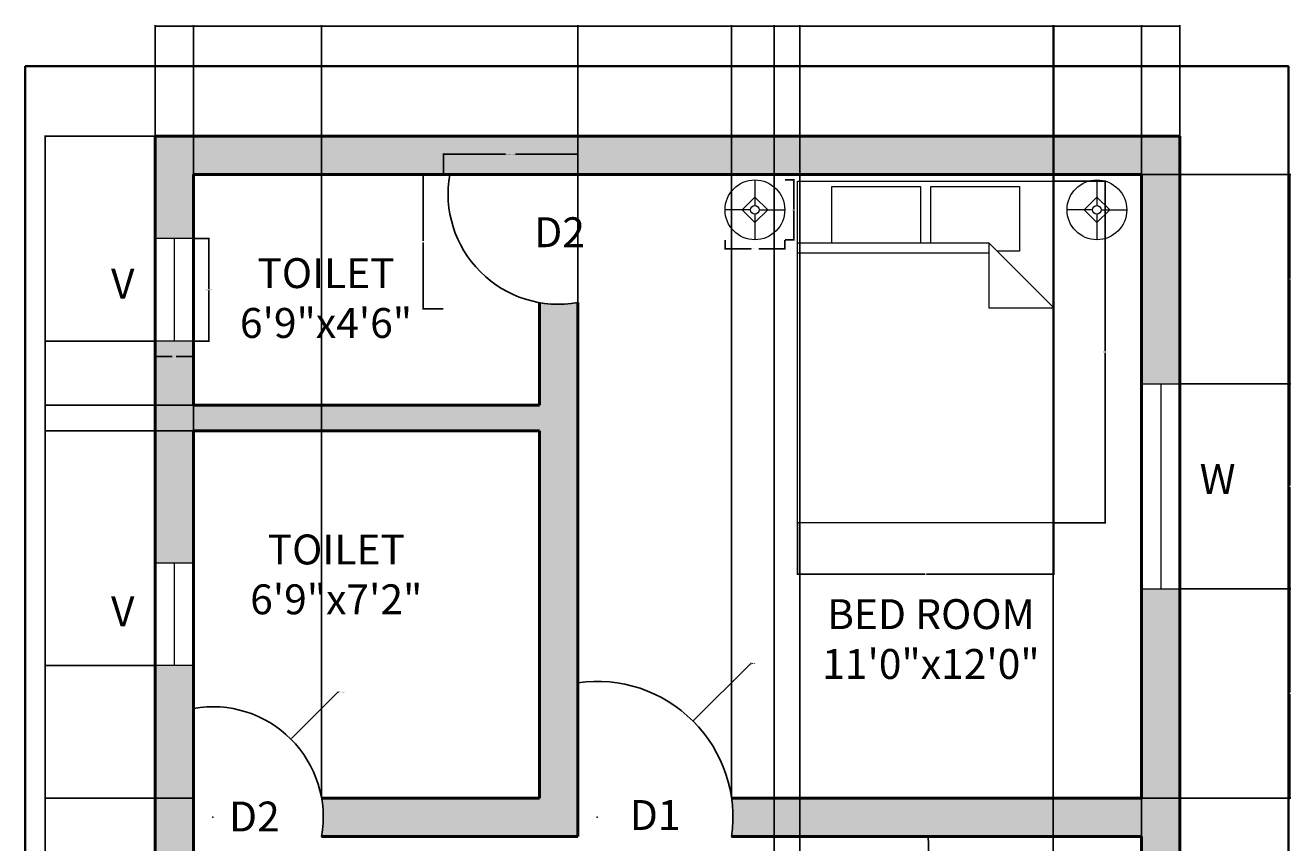
# Model space of a CAD drawing. Units: inches. Extents: x 1972 to 2269, y 1491 to 2023.
# Tile 3 of 3: x 1972 to 2269, y 1831 to 2023. Entities that reach past the tile are written whole.
import ezdxf

# ---------------------------------------------------------------- set-up
doc = ezdxf.new("R2010")
doc.units = ezdxf.units.IN
for name, color, linetype, lineweight in [('A-ANNO-DIMS', 2, 'Continuous', 18), ('A-ANNO-TEXT', 7, 'Continuous', 18), ('A-ANNO-TTLB', 7, 'Continuous', 35), ('A-AREA-IDEN', 7, 'Continuous', 25), ('A-DOOR', 3, 'Continuous', 25), ('A-FURN', 8, 'Continuous', 18), ('A-GLAZ', 4, 'Continuous', 18), ('A-WALL', 7, 'Continuous', 50)]:
    doc.layers.add(name, color=color, linetype=linetype, lineweight=lineweight)
doc.layers.add('A-WALL-PATT', color=18, linetype='Continuous', lineweight=13, true_color=0x000000)
doc.styles.get("Standard").update_dxf_attribs({"font": 'arial.ttf'})
doc.dimstyles.get("Standard").update_dxf_attribs({"dimtxt": 0.18, "dimasz": 0.18, "dimexe": 0.18, "dimexo": 0.0625, "dimgap": 0.09, "dimtad": 0, "dimtih": 1, "dimtoh": 1, "dimdec": 4, "dimzin": 0, "dimdsep": 46, "dimtxsty": 'Standard', "dimcen": 0.09, "dimadec": 0, "dimazin": 0, "dimtfac": 1, "dimtdec": 4, "dimtofl": 0, "dimtmove": 0, "dimatfit": 3, "dimfxl": 1, "dimtolj": 1, "dimtzin": 0, "dimarcsym": 0})

# ---------------------------------------------------------------- blocks, each defined once
blk = doc.blocks.new('Bed - Queen')
for p, q in [((0, -80.00003), (0, 0)), ((0, 0), (59.99999, 0)), ((59.99999, 0), (59.99999, -80.00003)), ((7.99999, -1.2), (28.79998, -1.2)), ((7.99999, -14.4), (7.99999, -1.2)), ((28.79998, -1.2), (28.79998, -14.4)), ((31.19999, -1.2), (51.99999, -1.2)), ((31.19999, -14.4), (31.19999, -1.2)), ((51.99999, -1.2), (51.99999, -16.4)), ((0, -14.4), (44.8, -14.4)), ((59.99999, -29.6), (44.8, -14.4)), ((44.8, -14.4), (44.8, -29.6)), ((44.8, -16.8), (0, -16.8)), ((51.99999, -16.4), (46.79936, -16.4)), ((44.8, -29.6), (59.99999, -29.6)), ((59.99999, -80.00003), (0, -80.00003))]:
    blk.add_line(p, q)
blk = doc.blocks.new('Lamp - Table')
for p, q in [((0, 7), (0, 1)), ((0, 3), (-3, 0)), ((3, 0), (0, 3)), ((-1, 0), (-7, 0)), ((-3, 0), (0, -3)), ((0, -3), (3, 0)), ((1, 0), (7, 0)), ((0, -1), (0, -7))]:
    blk.add_line(p, q)
for radius in [7, 1]:
    blk.add_circle((0, 0), radius)
blk = doc.blocks.new('VENT-24IN')
for p, q in [((9, 24), (0, 24)), ((4.5, 24), (4.5, 0)), ((9, 0), (0, 0))]:
    blk.add_line(p, q)
blk = doc.blocks.new('DOOR-SINGLE-30IN')
blk.add_line((0, 0), (0, 30))
blk.add_arc((4.5, 4.5), 25.89, 349.992, 100.008)
blk = doc.blocks.new('*D14')
at = {"layer": 'A-ANNO-DIMS', "color": 0, "lineweight": -2, "transparency": 16777216}
for p, q in [((2011.89, 1972.6), (2015.61, 1972.6)), ((2015.43, 1972.42), (2015.43, 1960.78)), ((2015.43, 1948.78), (2015.43, 1960.42)), ((2011.89, 1948.6), (2015.61, 1948.6))]:
    blk.add_line(p, q, dxfattribs=at)
at = {"layer": 'A-ANNO-DIMS', "color": 0, "transparency": 16777216}
for points in [[(2015.4, 1972.42), (2015.46, 1972.42), (2015.43, 1972.6)], [(2015.4, 1948.78), (2015.46, 1948.78), (2015.43, 1948.6)]]:
    blk.add_solid(points, dxfattribs=at)
at = {"layer": 'Defpoints', "color": 0, "transparency": 16777216}
for p in [(2011.83, 1972.6), (2015.43, 1972.6), (2011.83, 1948.6)]:
    blk.add_point(p, dxfattribs=at)
at = {"layer": 'A-ANNO-DIMS', "color": 0, "transparency": 16777216, "insert": (2015.43, 1960.6), "char_height": 0.18, "attachment_point": 5}
blk.add_mtext('\\A1;VENT 24 TYP.', dxfattribs=at)
blk = doc.blocks.new('*D15')
at = {"layer": 'A-ANNO-DIMS', "color": 0, "lineweight": -2, "transparency": 16777216}
for p, q in [((2002.83, 1948.54), (2002.83, 1944.82)), ((2011.83, 1948.54), (2011.83, 1944.82)), ((2003.01, 1945), (2006.87, 1945)), ((2011.65, 1945), (2007.78, 1945))]:
    blk.add_line(p, q, dxfattribs=at)
at = {"layer": 'A-ANNO-DIMS', "color": 0, "transparency": 16777216}
for points in [[(2003.01, 1945.03), (2003.01, 1944.97), (2002.83, 1945)], [(2011.65, 1945.03), (2011.65, 1944.97), (2011.83, 1945)]]:
    blk.add_solid(points, dxfattribs=at)
at = {"layer": 'Defpoints', "color": 0, "transparency": 16777216}
for p in [(2002.83, 1948.6), (2011.83, 1948.6), (2011.83, 1945)]:
    blk.add_point(p, dxfattribs=at)
at = {"layer": 'A-ANNO-DIMS', "color": 0, "transparency": 16777216, "insert": (2007.33, 1945), "char_height": 0.18, "attachment_point": 5}
blk.add_mtext('\\A1;9 TYP.', dxfattribs=at)
blk = doc.blocks.new('*D16')
at = {"layer": 'A-ANNO-DIMS', "color": 0, "lineweight": -2, "transparency": 16777216}
for p, q in [((2070.36, 1987.66), (2070.36, 1992.5)), ((2070.54, 1992.32), (2084.91, 1992.32)), ((2101.65, 1992.32), (2087.27, 1992.32)), ((2101.83, 1987.66), (2101.83, 1992.5))]:
    blk.add_line(p, q, dxfattribs=at)
at = {"layer": 'A-ANNO-DIMS', "color": 0, "transparency": 16777216}
for points in [[(2070.54, 1992.35), (2070.54, 1992.29), (2070.36, 1992.32)], [(2101.65, 1992.35), (2101.65, 1992.29), (2101.83, 1992.32)]]:
    blk.add_solid(points, dxfattribs=at)
at = {"layer": 'Defpoints', "color": 0, "transparency": 16777216}
for p in [(2070.36, 1992.32), (2070.36, 1987.6), (2101.83, 1987.6)]:
    blk.add_point(p, dxfattribs=at)
at = {"layer": 'A-ANNO-DIMS', "color": 0, "transparency": 16777216, "insert": (2086.09, 1992.32), "char_height": 0.18, "attachment_point": 5}
blk.add_mtext('\\A1;D2 SWING 31 TYP.', dxfattribs=at)
blk = doc.blocks.new('*D17')
at = {"layer": 'A-ANNO-DIMS', "color": 0, "lineweight": -2, "transparency": 16777216}
for p, q in [((2070.3, 1987.6), (2065.46, 1987.6)), ((2065.64, 1987.42), (2065.64, 1972.05)), ((2065.64, 1956.31), (2065.64, 1971.68)), ((2070.3, 1956.13), (2065.46, 1956.13))]:
    blk.add_line(p, q, dxfattribs=at)
at = {"layer": 'A-ANNO-DIMS', "color": 0, "transparency": 16777216}
for points in [[(2065.61, 1987.42), (2065.67, 1987.42), (2065.64, 1987.6)], [(2065.61, 1956.31), (2065.67, 1956.31), (2065.64, 1956.13)]]:
    blk.add_solid(points, dxfattribs=at)
at = {"layer": 'Defpoints', "color": 0, "transparency": 16777216}
for p in [(2070.36, 1987.6), (2065.64, 1956.13), (2070.36, 1956.13)]:
    blk.add_point(p, dxfattribs=at)
at = {"layer": 'A-ANNO-DIMS', "color": 0, "transparency": 16777216, "insert": (2065.64, 1971.86), "char_height": 0.18, "attachment_point": 5}
blk.add_mtext('\\A1;31 TYP.', dxfattribs=at)
blk = doc.blocks.new('*D18')
at = {"layer": 'A-ANNO-DIMS', "color": 0, "lineweight": -2, "transparency": 16777216}
for p, q in [((2136.29, 1972.26), (2136.29, 1970.05)), ((2150.29, 1972.26), (2150.29, 1970.05)), ((2136.47, 1970.23), (2142.39, 1970.23)), ((2150.11, 1970.23), (2144.19, 1970.23))]:
    blk.add_line(p, q, dxfattribs=at)
at = {"layer": 'A-ANNO-DIMS', "color": 0, "transparency": 16777216}
for points in [[(2136.47, 1970.26), (2136.47, 1970.2), (2136.29, 1970.23)], [(2150.11, 1970.26), (2150.11, 1970.2), (2150.29, 1970.23)]]:
    blk.add_solid(points, dxfattribs=at)
at = {"layer": 'Defpoints', "color": 0, "transparency": 16777216}
for p in [(2136.29, 1972.33), (2150.29, 1972.33), (2150.29, 1970.23)]:
    blk.add_point(p, dxfattribs=at)
at = {"layer": 'A-ANNO-DIMS', "color": 0, "transparency": 16777216, "insert": (2143.29, 1970.23), "char_height": 0.18, "attachment_point": 5}
blk.add_mtext('\\A1;LAMP 14 TYP.', dxfattribs=at)
blk = doc.blocks.new('*D19')
at = {"layer": 'A-ANNO-DIMS', "color": 0, "lineweight": -2, "transparency": 16777216}
for p, q in [((2150.35, 1986.33), (2152.57, 1986.33)), ((2152.39, 1986.15), (2152.39, 1979.51)), ((2152.39, 1972.51), (2152.39, 1979.14)), ((2150.35, 1972.33), (2152.57, 1972.33))]:
    blk.add_line(p, q, dxfattribs=at)
at = {"layer": 'A-ANNO-DIMS', "color": 0, "transparency": 16777216}
for points in [[(2152.36, 1986.15), (2152.42, 1986.15), (2152.39, 1986.33)], [(2152.36, 1972.51), (2152.42, 1972.51), (2152.39, 1972.33)]]:
    blk.add_solid(points, dxfattribs=at)
at = {"layer": 'Defpoints', "color": 0, "transparency": 16777216}
for p in [(2150.29, 1986.33), (2152.39, 1986.33), (2150.29, 1972.33)]:
    blk.add_point(p, dxfattribs=at)
at = {"layer": 'A-ANNO-DIMS', "color": 0, "transparency": 16777216, "insert": (2152.39, 1979.33), "char_height": 0.18, "attachment_point": 5}
blk.add_mtext('\\A1;14 TYP.', dxfattribs=at)
blk = doc.blocks.new('*D20')
at = {"layer": 'A-ANNO-DIMS', "color": 0, "lineweight": -2, "transparency": 16777216}
for p, q in [((2213.34, 1986.02), (2225.46, 1986.02)), ((2225.28, 1985.84), (2225.28, 1946.2)), ((2225.28, 1906.2), (2225.28, 1945.83)), ((2213.34, 1906.02), (2225.46, 1906.02))]:
    blk.add_line(p, q, dxfattribs=at)
at = {"layer": 'A-ANNO-DIMS', "color": 0, "transparency": 16777216}
for points in [[(2225.25, 1985.84), (2225.31, 1985.84), (2225.28, 1986.02)], [(2225.25, 1906.2), (2225.31, 1906.2), (2225.28, 1906.02)]]:
    blk.add_solid(points, dxfattribs=at)
at = {"layer": 'Defpoints', "color": 0, "transparency": 16777216}
for p in [(2213.28, 1986.02), (2225.28, 1986.02), (2213.28, 1906.02)]:
    blk.add_point(p, dxfattribs=at)
at = {"layer": 'A-ANNO-DIMS', "color": 0, "transparency": 16777216, "insert": (2225.28, 1946.02), "char_height": 0.18, "attachment_point": 5}
blk.add_mtext('\\A1;BED 80', dxfattribs=at)
blk = doc.blocks.new('*D21')
at = {"layer": 'A-ANNO-DIMS', "color": 0, "lineweight": -2, "transparency": 16777216}
for p, q in [((2153.28, 1905.95), (2153.28, 1893.84)), ((2213.28, 1905.95), (2213.28, 1893.84)), ((2153.46, 1894.02), (2183.06, 1894.02)), ((2213.1, 1894.02), (2183.49, 1894.02))]:
    blk.add_line(p, q, dxfattribs=at)
at = {"layer": 'A-ANNO-DIMS', "color": 0, "transparency": 16777216}
for points in [[(2153.46, 1894.05), (2153.46, 1893.99), (2153.28, 1894.02)], [(2213.1, 1894.05), (2213.1, 1893.99), (2213.28, 1894.02)]]:
    blk.add_solid(points, dxfattribs=at)
at = {"layer": 'Defpoints', "color": 0, "transparency": 16777216}
for p in [(2153.28, 1906.02), (2213.28, 1906.02), (2213.28, 1894.02)]:
    blk.add_point(p, dxfattribs=at)
at = {"layer": 'A-ANNO-DIMS', "color": 0, "transparency": 16777216, "insert": (2183.28, 1894.02), "char_height": 0.18, "attachment_point": 5}
blk.add_mtext('\\A1;60', dxfattribs=at)
blk = doc.blocks.new('*D28')
at = {"layer": 'A-ANNO-DIMS', "color": 0, "lineweight": -2, "transparency": 16777216}
for p, q in [((2002.83, 1996.66), (2002.83, 2022.53)), ((2003.01, 2022.35), (2122.54, 2022.35)), ((2242.65, 2022.35), (2123.12, 2022.35)), ((2242.83, 1790.66), (2242.83, 2022.53))]:
    blk.add_line(p, q, dxfattribs=at)
at = {"layer": 'A-ANNO-DIMS', "color": 0, "transparency": 16777216}
for points in [[(2003.01, 2022.38), (2003.01, 2022.32), (2002.83, 2022.35)], [(2242.65, 2022.38), (2242.65, 2022.32), (2242.83, 2022.35)]]:
    blk.add_solid(points, dxfattribs=at)
at = {"layer": 'Defpoints', "color": 0, "transparency": 16777216}
for p in [(2242.83, 2022.35), (2002.83, 1996.6), (2242.83, 1790.6)]:
    blk.add_point(p, dxfattribs=at)
at = {"layer": 'A-ANNO-DIMS', "color": 0, "transparency": 16777216, "insert": (2122.83, 2022.35), "char_height": 0.18, "attachment_point": 5}
blk.add_mtext('\\A1;240', dxfattribs=at)
blk = doc.blocks.new('*D29')
at = {"layer": 'A-ANNO-DIMS', "color": 0, "lineweight": -2, "transparency": 16777216}
for p, q in [((2002.76, 1996.6), (1976.9, 1996.6)), ((1977.08, 1996.42), (1977.08, 1756.78)), ((1977.08, 1516.78), (1977.08, 1756.42)), ((2002.76, 1516.6), (1976.9, 1516.6))]:
    blk.add_line(p, q, dxfattribs=at)
at = {"layer": 'A-ANNO-DIMS', "color": 0, "transparency": 16777216}
for points in [[(1977.05, 1996.42), (1977.11, 1996.42), (1977.08, 1996.6)], [(1977.05, 1516.78), (1977.11, 1516.78), (1977.08, 1516.6)]]:
    blk.add_solid(points, dxfattribs=at)
at = {"layer": 'Defpoints', "color": 0, "transparency": 16777216}
for p in [(1977.08, 1996.6), (2002.83, 1996.6), (2002.83, 1516.6)]:
    blk.add_point(p, dxfattribs=at)
at = {"layer": 'A-ANNO-DIMS', "color": 0, "transparency": 16777216, "insert": (1977.08, 1756.6), "char_height": 0.18, "attachment_point": 5}
blk.add_mtext('\\A1;480', dxfattribs=at)
blk = doc.blocks.new('*D31')
at = {"layer": 'A-ANNO-DIMS', "color": 0, "lineweight": -2, "transparency": 16777216}
for p, q in [((2011.76, 1933.6), (1976.9, 1933.6)), ((1977.08, 1933.42), (1977.08, 1930.78)), ((1977.08, 1927.78), (1977.08, 1930.42)), ((2011.76, 1927.6), (1976.9, 1927.6))]:
    blk.add_line(p, q, dxfattribs=at)
at = {"layer": 'A-ANNO-DIMS', "color": 0, "transparency": 16777216}
for points in [[(1977.05, 1933.42), (1977.11, 1933.42), (1977.08, 1933.6)], [(1977.05, 1927.78), (1977.11, 1927.78), (1977.08, 1927.6)]]:
    blk.add_solid(points, dxfattribs=at)
at = {"layer": 'Defpoints', "color": 0, "transparency": 16777216}
for p in [(2011.83, 1933.6), (1977.08, 1927.6), (2011.83, 1927.6)]:
    blk.add_point(p, dxfattribs=at)
at = {"layer": 'A-ANNO-DIMS', "color": 0, "transparency": 16777216, "insert": (1977.08, 1930.6), "char_height": 0.18, "attachment_point": 5}
blk.add_mtext('\\A1;6', dxfattribs=at)
blk = doc.blocks.new('*D32')
at = {"layer": 'A-ANNO-DIMS', "color": 0, "lineweight": -2, "transparency": 16777216}
for p, q in [((2242.89, 1938.6), (2268.76, 1938.6)), ((2268.58, 1938.42), (2268.58, 1914.78)), ((2268.58, 1890.78), (2268.58, 1914.42)), ((2242.89, 1890.6), (2268.76, 1890.6))]:
    blk.add_line(p, q, dxfattribs=at)
at = {"layer": 'A-ANNO-DIMS', "color": 0, "transparency": 16777216}
for points in [[(2268.55, 1938.42), (2268.61, 1938.42), (2268.58, 1938.6)], [(2268.55, 1890.78), (2268.61, 1890.78), (2268.58, 1890.6)]]:
    blk.add_solid(points, dxfattribs=at)
at = {"layer": 'Defpoints', "color": 0, "transparency": 16777216}
for p in [(2242.83, 1938.6), (2268.58, 1938.6), (2242.83, 1890.6)]:
    blk.add_point(p, dxfattribs=at)
at = {"layer": 'A-ANNO-DIMS', "color": 0, "transparency": 16777216, "insert": (2268.58, 1914.6), "char_height": 0.18, "attachment_point": 5}
blk.add_mtext('\\A1;48', dxfattribs=at)
blk = doc.blocks.new('*D33')
at = {"layer": 'A-ANNO-DIMS', "color": 0, "lineweight": -2, "transparency": 16777216}
for p, q in [((2242.89, 1890.6), (2268.76, 1890.6)), ((2268.58, 1890.42), (2268.58, 1866.28)), ((2268.58, 1841.78), (2268.58, 1865.92)), ((2233.89, 1841.6), (2268.76, 1841.6))]:
    blk.add_line(p, q, dxfattribs=at)
at = {"layer": 'A-ANNO-DIMS', "color": 0, "transparency": 16777216}
for points in [[(2268.55, 1890.42), (2268.61, 1890.42), (2268.58, 1890.6)], [(2268.55, 1841.78), (2268.61, 1841.78), (2268.58, 1841.6)]]:
    blk.add_solid(points, dxfattribs=at)
at = {"layer": 'Defpoints', "color": 0, "transparency": 16777216}
for p in [(2242.83, 1890.6), (2268.58, 1890.6), (2233.83, 1841.6)]:
    blk.add_point(p, dxfattribs=at)
at = {"layer": 'A-ANNO-DIMS', "color": 0, "transparency": 16777216, "insert": (2268.58, 1866.1), "char_height": 0.18, "attachment_point": 5}
blk.add_mtext('\\A1;49', dxfattribs=at)
blk = doc.blocks.new('*D34')
at = {"layer": 'A-ANNO-DIMS', "color": 0, "lineweight": -2, "transparency": 16777216}
for p, q in [((2233.89, 1987.6), (2268.76, 1987.6)), ((2268.58, 1987.42), (2268.58, 1963.28)), ((2268.58, 1938.78), (2268.58, 1962.92)), ((2242.89, 1938.6), (2268.76, 1938.6))]:
    blk.add_line(p, q, dxfattribs=at)
at = {"layer": 'A-ANNO-DIMS', "color": 0, "transparency": 16777216}
for points in [[(2268.55, 1987.42), (2268.61, 1987.42), (2268.58, 1987.6)], [(2268.55, 1938.78), (2268.61, 1938.78), (2268.58, 1938.6)]]:
    blk.add_solid(points, dxfattribs=at)
at = {"layer": 'Defpoints', "color": 0, "transparency": 16777216}
for p in [(2233.83, 1987.6), (2268.58, 1987.6), (2242.83, 1938.6)]:
    blk.add_point(p, dxfattribs=at)
at = {"layer": 'A-ANNO-DIMS', "color": 0, "transparency": 16777216, "insert": (2268.58, 1963.1), "char_height": 0.18, "attachment_point": 5}
blk.add_mtext('\\A1;49', dxfattribs=at)
blk = doc.blocks.new('*D38')
at = {"layer": 'A-ANNO-DIMS', "color": 0, "lineweight": -2, "transparency": 16777216}
for p, q in [((2002.76, 1872.6), (1976.9, 1872.6)), ((1977.08, 1872.42), (1977.08, 1857.28)), ((1977.08, 1841.78), (1977.08, 1856.92)), ((2011.76, 1841.6), (1976.9, 1841.6))]:
    blk.add_line(p, q, dxfattribs=at)
at = {"layer": 'A-ANNO-DIMS', "color": 0, "transparency": 16777216}
for points in [[(1977.05, 1872.42), (1977.11, 1872.42), (1977.08, 1872.6)], [(1977.05, 1841.78), (1977.11, 1841.78), (1977.08, 1841.6)]]:
    blk.add_solid(points, dxfattribs=at)
at = {"layer": 'Defpoints', "color": 0, "transparency": 16777216}
for p in [(1977.08, 1872.6), (2002.83, 1872.6), (2011.83, 1841.6)]:
    blk.add_point(p, dxfattribs=at)
at = {"layer": 'A-ANNO-DIMS', "color": 0, "transparency": 16777216, "insert": (1977.08, 1857.1), "char_height": 0.18, "attachment_point": 5}
blk.add_mtext('\\A1;31', dxfattribs=at)
blk = doc.blocks.new('*D39')
at = {"layer": 'A-ANNO-DIMS', "color": 0, "lineweight": -2, "transparency": 16777216}
for p, q in [((2002.76, 1948.6), (1976.9, 1948.6)), ((1977.08, 1948.42), (1977.08, 1941.28)), ((1977.08, 1933.78), (1977.08, 1940.92)), ((2011.76, 1933.6), (1976.9, 1933.6))]:
    blk.add_line(p, q, dxfattribs=at)
at = {"layer": 'A-ANNO-DIMS', "color": 0, "transparency": 16777216}
for points in [[(1977.05, 1948.42), (1977.11, 1948.42), (1977.08, 1948.6)], [(1977.05, 1933.78), (1977.11, 1933.78), (1977.08, 1933.6)]]:
    blk.add_solid(points, dxfattribs=at)
at = {"layer": 'Defpoints', "color": 0, "transparency": 16777216}
for p in [(1977.08, 1948.6), (2002.83, 1948.6), (2011.83, 1933.6)]:
    blk.add_point(p, dxfattribs=at)
at = {"layer": 'A-ANNO-DIMS', "color": 0, "transparency": 16777216, "insert": (1977.08, 1941.1), "char_height": 0.18, "attachment_point": 5}
blk.add_mtext('\\A1;15', dxfattribs=at)
blk = doc.blocks.new('*D43')
at = {"layer": 'A-ANNO-DIMS', "color": 0, "lineweight": -2, "transparency": 16777216}
for p, q in [((2101.83, 1841.66), (2101.83, 2022.53)), ((2102.01, 2022.35), (2119.61, 2022.35)), ((2137.65, 2022.35), (2120.05, 2022.35)), ((2137.83, 1841.66), (2137.83, 2022.53))]:
    blk.add_line(p, q, dxfattribs=at)
at = {"layer": 'A-ANNO-DIMS', "color": 0, "transparency": 16777216}
for points in [[(2102.01, 2022.38), (2102.01, 2022.32), (2101.83, 2022.35)], [(2137.65, 2022.38), (2137.65, 2022.32), (2137.83, 2022.35)]]:
    blk.add_solid(points, dxfattribs=at)
at = {"layer": 'Defpoints', "color": 0, "transparency": 16777216}
for p in [(2137.83, 2022.35), (2101.83, 1841.6), (2137.83, 1841.6)]:
    blk.add_point(p, dxfattribs=at)
at = {"layer": 'A-ANNO-DIMS', "color": 0, "transparency": 16777216, "insert": (2119.83, 2022.35), "char_height": 0.18, "attachment_point": 5}
blk.add_mtext('\\A1;36', dxfattribs=at)
blk = doc.blocks.new('*D44')
at = {"layer": 'A-ANNO-DIMS', "color": 0, "lineweight": -2, "transparency": 16777216}
for p, q in [((2011.83, 1841.66), (2011.83, 2022.53)), ((2012.01, 2022.35), (2026.61, 2022.35)), ((2041.65, 2022.35), (2027.05, 2022.35)), ((2041.83, 1841.66), (2041.83, 2022.53))]:
    blk.add_line(p, q, dxfattribs=at)
at = {"layer": 'A-ANNO-DIMS', "color": 0, "transparency": 16777216}
for points in [[(2012.01, 2022.38), (2012.01, 2022.32), (2011.83, 2022.35)], [(2041.65, 2022.38), (2041.65, 2022.32), (2041.83, 2022.35)]]:
    blk.add_solid(points, dxfattribs=at)
at = {"layer": 'Defpoints', "color": 0, "transparency": 16777216}
for p in [(2041.83, 2022.35), (2011.83, 1841.6), (2041.83, 1841.6)]:
    blk.add_point(p, dxfattribs=at)
at = {"layer": 'A-ANNO-DIMS', "color": 0, "transparency": 16777216, "insert": (2026.83, 2022.35), "char_height": 0.18, "attachment_point": 5}
blk.add_mtext('\\A1;30', dxfattribs=at)
blk = doc.blocks.new('*D52')
at = {"layer": 'A-ANNO-DIMS', "color": 0, "lineweight": -2, "transparency": 16777216}
for p, q in [((2213.15, 1795.78), (2213.15, 2022.53)), ((2213.33, 2022.35), (2223.02, 2022.35)), ((2233.65, 2022.35), (2223.96, 2022.35)), ((2233.83, 1795.78), (2233.83, 2022.53))]:
    blk.add_line(p, q, dxfattribs=at)
at = {"layer": 'A-ANNO-DIMS', "color": 0, "transparency": 16777216}
for points in [[(2213.33, 2022.38), (2213.33, 2022.32), (2213.15, 2022.35)], [(2233.65, 2022.38), (2233.65, 2022.32), (2233.83, 2022.35)]]:
    blk.add_solid(points, dxfattribs=at)
at = {"layer": 'Defpoints', "color": 0, "transparency": 16777216}
for p in [(2233.83, 2022.35), (2213.15, 1795.72), (2233.83, 1795.72)]:
    blk.add_point(p, dxfattribs=at)
at = {"layer": 'A-ANNO-DIMS', "color": 0, "transparency": 16777216, "insert": (2223.49, 2022.35), "char_height": 0.18, "attachment_point": 5}
blk.add_mtext('\\A1;20.673', dxfattribs=at)
blk = doc.blocks.new('*D55')
at = {"layer": 'A-ANNO-DIMS', "color": 0, "lineweight": -2, "transparency": 16777216}
for p, q in [((2213.28, 1986.08), (2213.28, 2022.53)), ((2213.46, 2022.35), (2223.15, 2022.35)), ((2233.65, 2022.35), (2223.95, 2022.35)), ((2233.83, 1987.66), (2233.83, 2022.53))]:
    blk.add_line(p, q, dxfattribs=at)
at = {"layer": 'A-ANNO-DIMS', "color": 0, "transparency": 16777216}
for points in [[(2213.46, 2022.38), (2213.46, 2022.32), (2213.28, 2022.35)], [(2233.65, 2022.38), (2233.65, 2022.32), (2233.83, 2022.35)]]:
    blk.add_solid(points, dxfattribs=at)
at = {"layer": 'Defpoints', "color": 0, "transparency": 16777216}
for p in [(2213.28, 2022.35), (2213.28, 1986.02), (2233.83, 1987.6)]:
    blk.add_point(p, dxfattribs=at)
at = {"layer": 'A-ANNO-DIMS', "color": 0, "transparency": 16777216, "insert": (2223.55, 2022.35), "char_height": 0.18, "attachment_point": 5}
blk.add_mtext('\\A1;20.55', dxfattribs=at)
blk = doc.blocks.new('*D56')
at = {"layer": 'A-ANNO-DIMS', "color": 0, "lineweight": -2, "transparency": 16777216}
for p, q in [((2011.83, 1832.54), (2011.83, 1490.67)), ((2147.83, 1796.54), (2147.83, 1490.67)), ((2012.01, 1490.85), (2079.55, 1490.85)), ((2147.65, 1490.85), (2080.11, 1490.85))]:
    blk.add_line(p, q, dxfattribs=at)
at = {"layer": 'A-ANNO-DIMS', "color": 0, "transparency": 16777216}
for points in [[(2012.01, 1490.88), (2012.01, 1490.82), (2011.83, 1490.85)], [(2147.65, 1490.88), (2147.65, 1490.82), (2147.83, 1490.85)]]:
    blk.add_solid(points, dxfattribs=at)
at = {"layer": 'Defpoints', "color": 0, "transparency": 16777216}
for p in [(2011.83, 1832.6), (2147.83, 1796.6), (2147.83, 1490.85)]:
    blk.add_point(p, dxfattribs=at)
at = {"layer": 'A-ANNO-DIMS', "color": 0, "transparency": 16777216, "insert": (2079.83, 1490.85), "char_height": 0.18, "attachment_point": 5}
blk.add_mtext('\\A1;136', dxfattribs=at)
blk = doc.blocks.new('*D57')
at = {"layer": 'A-ANNO-DIMS', "color": 0, "lineweight": -2, "transparency": 16777216}
for p, q in [((2147.83, 1796.66), (2147.83, 2022.53)), ((2148.01, 2022.35), (2150.68, 2022.35)), ((2153.65, 2022.35), (2150.98, 2022.35)), ((2153.83, 1796.66), (2153.83, 2022.53))]:
    blk.add_line(p, q, dxfattribs=at)
at = {"layer": 'A-ANNO-DIMS', "color": 0, "transparency": 16777216}
for points in [[(2148.01, 2022.38), (2148.01, 2022.32), (2147.83, 2022.35)], [(2153.65, 2022.38), (2153.65, 2022.32), (2153.83, 2022.35)]]:
    blk.add_solid(points, dxfattribs=at)
at = {"layer": 'Defpoints', "color": 0, "transparency": 16777216}
for p in [(2153.83, 2022.35), (2147.83, 1796.6), (2153.83, 1796.6)]:
    blk.add_point(p, dxfattribs=at)
at = {"layer": 'A-ANNO-DIMS', "color": 0, "transparency": 16777216, "insert": (2150.83, 2022.35), "char_height": 0.18, "attachment_point": 5}
blk.add_mtext('\\A1;6', dxfattribs=at)
blk = doc.blocks.new('*D59')
at = {"layer": 'A-ANNO-DIMS', "color": 0, "lineweight": -2, "transparency": 16777216}
for p, q in [((2045.62, 1866.4), (2034.76, 1855.54)), ((2045.8, 1866.4), (2045.62, 1866.4)), ((2016.33, 1837.01), (2016.33, 1837.19)), ((2016.24, 1837.1), (2016.42, 1837.1))]:
    blk.add_line(p, q, dxfattribs=at)
at = {"layer": 'A-ANNO-DIMS', "color": 0, "transparency": 16777216}
blk.add_solid([(2034.74, 1855.56), (2034.78, 1855.52), (2034.64, 1855.41)], dxfattribs=at)
at = {"layer": 'Defpoints', "color": 0, "transparency": 16777216}
for p in [(2034.64, 1855.41), (2016.33, 1837.1)]:
    blk.add_point(p, dxfattribs=at)
at = {"layer": 'A-ANNO-DIMS', "color": 0, "transparency": 16777216, "insert": (2046.55, 1866.4), "char_height": 0.18, "attachment_point": 5}
blk.add_mtext('\\A1;2X R25.894', dxfattribs=at)
blk = doc.blocks.new('*D61')
at = {"layer": 'A-ANNO-DIMS', "color": 0, "lineweight": -2, "transparency": 16777216}
for p, q in [((2142.33, 1873.1), (2128.95, 1859.73)), ((2142.51, 1873.1), (2142.33, 1873.1)), ((2106.33, 1837.01), (2106.33, 1837.19)), ((2106.24, 1837.1), (2106.42, 1837.1))]:
    blk.add_line(p, q, dxfattribs=at)
at = {"layer": 'A-ANNO-DIMS', "color": 0, "transparency": 16777216}
blk.add_solid([(2128.93, 1859.75), (2128.98, 1859.7), (2128.83, 1859.6)], dxfattribs=at)
at = {"layer": 'Defpoints', "color": 0, "transparency": 16777216}
for p in [(2128.83, 1859.6), (2106.33, 1837.1)]:
    blk.add_point(p, dxfattribs=at)
at = {"layer": 'A-ANNO-DIMS', "color": 0, "transparency": 16777216, "insert": (2142.99, 1873.1), "char_height": 0.18, "attachment_point": 5}
blk.add_mtext('\\A1;R31.82', dxfattribs=at)

msp = doc.modelspace()

# ---------------------------------------------------------------- hatches: boundary and pattern name
at = {"layer": 'A-WALL-PATT'}
h = msp.add_hatch(color=256, dxfattribs=at)
h.dxf.hatch_style = 1
h.paths.add_polyline_path([(2242.8266, 1996.5987), (2002.8266, 1996.5987), (2002.8266, 1972.5987), (2011.8266, 1972.5987), (2011.8266, 1987.5987), (2092.8266, 1987.5987), (2101.8266, 1987.5987), (2233.8266, 1987.5987), (2233.8266, 1938.5987), (2242.8266, 1938.5987)])
h.paths.add_polyline_path([(2101.8266, 1957.5987, -0.08755883), (2092.8266, 1957.5987), (2092.8266, 1933.5987), (2011.8266, 1933.5987), (2011.8266, 1948.5987), (2002.8266, 1948.5987), (2002.8266, 1896.5987), (2011.8266, 1896.5987), (2011.8266, 1927.5987), (2092.8266, 1927.5987), (2092.8266, 1841.5987), (2041.8266, 1841.5987, -0.08755883), (2041.8266, 1832.5987), (2092.8266, 1832.5987), (2101.8266, 1832.5987), (2101.8266, 1868.5987)])
h.paths.add_polyline_path([(2242.8266, 1890.5987), (2233.8266, 1890.5987), (2233.8266, 1841.5987), (2137.8266, 1841.5987, -0.07106781), (2137.8266, 1832.5987), (2147.8266, 1832.5987), (2183.8266, 1832.5987), (2233.8266, 1832.5987), (2233.8266, 1790.5987), (2242.8266, 1790.5987)])
h.paths.add_polyline_path([(2011.8266, 1832.5987), (2011.8266, 1862.5987), (2011.8266, 1872.5987), (2002.8266, 1872.5987), (2002.8266, 1516.5987), (2022.3266, 1516.5987), (2022.3266, 1525.5987), (2011.8266, 1525.5987), (2011.8266, 1679.5987), (2092.8266, 1679.5987), (2092.8266, 1643.5987), (2092.8266, 1573.5987), (2101.8266, 1573.5987), (2101.8266, 1643.5987), (2101.8266, 1679.5987), (2101.8266, 1688.5987), (2011.8266, 1688.5987)])
h.paths.add_polyline_path([(2140.2493, 1525.5987), (2101.8266, 1525.5987), (2092.8266, 1525.5987), (2082.3266, 1525.5987), (2082.3266, 1516.5987), (2140.2493, 1516.5987)])
h.paths.add_polyline_path([(2242.8266, 1568.0987), (2233.8266, 1568.0987), (2233.8266, 1525.5987), (2233.8266, 1516.5987), (2242.8266, 1516.5987)])
h.paths.add_polyline_path([(2242.8266, 1730.5987), (2233.8266, 1730.5987), (2233.8266, 1688.5987), (2223.8266, 1688.5987), (2223.8266, 1679.5987), (2233.8266, 1679.5987), (2233.8266, 1628.0987), (2242.8266, 1628.0987)])
h.paths.add_polyline_path([(2163.8266, 1688.5987), (2153.8266, 1688.5987), (2153.8266, 1796.5987, -0.04536102), (2147.8266, 1796.5987), (2147.8266, 1688.5987), (2147.8266, 1679.5987), (2153.8266, 1679.5987), (2163.8266, 1679.5987)])

# ---------------------------------------------------------------- linework, layer by layer
at = {"layer": 'A-ANNO-TTLB'}
msp.add_lwpolyline([(1972.4438, 2012.9515), (2268.2203, 2012.9515), (2268.2203, 1493.2355), (1972.4438, 1493.2355)], close=True, dxfattribs=at)
at = {"layer": 'A-DOOR'}
for p, q in [((2101.8266, 1832.5987), (2101.8266, 1868.5987)), ((2147.8266, 1832.5987), (2183.8266, 1832.5987))]:
    msp.add_line(p, q, dxfattribs=at)
for centre, radius, start, end in [((2106.3266, 1837.0987), 31.8198, 351.869898, 98.130102), ((2150.8266, 1829.5987), 33.1361, 264.805571, 5.194429)]:
    msp.add_arc(centre, radius, start, end, dxfattribs=at)
at = {"layer": 'A-GLAZ'}
for p, q in [((2233.8266, 1938.5987), (2242.8266, 1938.5987)), ((2238.3266, 1938.5987), (2238.3266, 1890.5987)), ((2233.8266, 1890.5987), (2242.8266, 1890.5987))]:
    msp.add_line(p, q, dxfattribs=at)
at = {"layer": 'A-WALL'}
for p, q in [((2002.8266, 1996.5987), (2242.8266, 1996.5987)), ((2002.8266, 1516.5987), (2002.8266, 1996.5987)), ((2242.8266, 1996.5987), (2242.8266, 1516.5987)), ((2011.8266, 1987.5987), (2092.8266, 1987.5987)), ((2011.8266, 1933.5987), (2011.8266, 1987.5987)), ((2092.8266, 1987.5987), (2101.8266, 1987.5987)), ((2101.8266, 1987.5987), (2233.8266, 1987.5987)), ((2233.8266, 1987.5987), (2233.8266, 1841.5987)), ((2092.8266, 1933.5987), (2092.8266, 1957.5987)), ((2101.8266, 1841.5987), (2101.8266, 1957.5987)), ((2011.8266, 1933.5987), (2092.8266, 1933.5987)), ((2011.8266, 1927.5987), (2092.8266, 1927.5987)), ((2011.8266, 1841.5987), (2011.8266, 1927.5987)), ((2092.8266, 1841.5987), (2092.8266, 1927.5987)), ((2011.8266, 1841.5987), (2011.8266, 1832.5987)), ((2041.8266, 1841.5987), (2092.8266, 1841.5987)), ((2101.8266, 1841.5987), (2101.8266, 1832.5987)), ((2137.8266, 1841.5987), (2233.8266, 1841.5987)), ((2011.8266, 1688.5987), (2011.8266, 1832.5987)), ((2041.8266, 1832.5987), (2092.8266, 1832.5987)), ((2092.8266, 1832.5987), (2101.8266, 1832.5987)), ((2137.8266, 1832.5987), (2147.8266, 1832.5987)), ((2147.8266, 1832.5987), (2153.8266, 1832.5987)), ((2153.8266, 1832.5987), (2233.8266, 1832.5987)), ((2233.8266, 1832.5987), (2233.8266, 1688.5987))]:
    msp.add_line(p, q, dxfattribs=at)

# ---------------------------------------------------------------- block references
at = {"layer": 'A-DOOR', "extrusion": (0, 0, -1), "zscale": -1, "rotation": 270.0000000000012}
msp.add_blockref('DOOR-SINGLE-30IN', (-2101.8263, 1987.5983), dxfattribs=at)
at = {"layer": 'A-DOOR'}
msp.add_blockref('DOOR-SINGLE-30IN', (2011.827, 1832.599), dxfattribs=at)
at = {"layer": 'A-FURN'}
for name, p in [('Lamp - Table', (2143.2904, 1979.3252)), ('Bed - Queen', (2153.2751, 1986.0159)), ('Lamp - Table', (2223.3812, 1979.3252))]:
    msp.add_blockref(name, p, dxfattribs=at)
at = {"layer": 'A-GLAZ'}
for p in [(2002.827, 1948.599), (2002.827, 1872.599)]:
    msp.add_blockref('VENT-24IN', p, dxfattribs=at)

# ---------------------------------------------------------------- texts
at = {"layer": 'A-ANNO-TEXT', "char_height": 7, "attachment_point": 1}
for s, width, insert in [('\\pxqc;D2', 12.170588, (2091.4715, 1977.5816)), ('\\pxqc;V', 9.762187, (1990.3766, 1965.5369)), ('\\pxqc;W', 23.220679, (2240.0281, 1919.7789)), ('\\pxqc;V', 9.762187, (1990.3766, 1888.8227)), ('\\pxqc;D2', 16.79729, (2017.6829, 1840.7697)), ('\\pxqc;D1', 14.325496, (2112.7708, 1841.1201))]:
    msp.add_mtext_dynamic_manual_height_columns(s, width=width, gutter_width=12.5, heights=[0], dxfattribs=dict(at, insert=insert))
at = {"layer": 'A-AREA-IDEN', "char_height": 7, "attachment_point": 1}
for s, width, insert in [('\\pxqc;{\\fArial|b1|i0|c0|p34;TOILET\\P6\'9"x4\'6"}', 55.386026, (2015.1684, 1968.0066)), ('\\pxqc;{\\fArial|b1|i0|c0|p34;TOILET\\P6\'9"x7\'2"}', 60.965596, (2014.7799, 1903.2987)), ('\\pxqc;{\\fArial|b1|i0|c0|p34;BED ROOM\\P11\'0"x12\'0"}', 75.996366, (2146.5141, 1888.1626))]:
    msp.add_mtext_dynamic_manual_height_columns(s, width=width, gutter_width=12.5, heights=[0], dxfattribs=dict(at, insert=insert))

# ---------------------------------------------------------------- dimensions: what is measured, and where the dimension line sits
at = {"layer": 'A-ANNO-DIMS'}
for base, p1, p2, override, picture, middle in [((2242.8266, 2022.3487), (2002.8266, 1996.5987), (2242.8266, 1790.5987), {"dimdec": 0, "dimlfac": 1, "dimrnd": 0, "dimzin": 0, "dimdsep": 46, "dimlunit": 2}, '*D28', (2122.8266, 2022.3487)), ((2041.8266, 2022.3487), (2011.8266, 1841.5987), (2041.8266, 1841.5987), {"dimdec": 0, "dimlfac": 1, "dimrnd": 0, "dimzin": 0, "dimdsep": 46, "dimlunit": 2}, '*D44', (2026.8266, 2022.3487)), ((2137.8266, 2022.3487), (2101.8266, 1841.5987), (2137.8266, 1841.5987), {"dimdec": 0, "dimlfac": 1, "dimrnd": 0, "dimzin": 0, "dimdsep": 46, "dimlunit": 2}, '*D43', (2119.8266, 2022.3487)), ((2153.8266, 2022.3487), (2147.8266, 1796.5987), (2153.8266, 1796.5987), {"dimdec": 0, "dimlfac": 1, "dimrnd": 0, "dimzin": 0, "dimdsep": 46, "dimlunit": 2}, '*D57', (2150.8266, 2022.3487)), ((2233.8266, 2022.3487), (2213.1538, 1795.7186), (2233.8266, 1795.7186), {"dimdec": 3, "dimlfac": 1, "dimrnd": 0, "dimzin": 0, "dimdsep": 46, "dimlunit": 2}, '*D52', (2223.4902, 2022.3487)), ((2213.2751, 2022.3487), (2233.8266, 1987.5987), (2213.2751, 1986.0159), {"dimdec": 2, "dimlfac": 1, "dimrnd": 0, "dimzin": 0, "dimdsep": 46, "dimlunit": 2}, '*D55', (2223.5508, 2022.3487)), ((2213.2751, 1894.0159), (2153.2751, 1906.0159), (2213.2751, 1906.0159), {"dimdec": 0, "dimlfac": 1, "dimrnd": 0, "dimzin": 0, "dimdsep": 46, "dimlunit": 2}, '*D21', (2183.2751, 1894.0159)), ((2147.8266, 1490.8487), (2011.8266, 1832.5987), (2147.8266, 1796.5987), {"dimdec": 0, "dimlfac": 1, "dimrnd": 0, "dimzin": 0, "dimdsep": 46, "dimlunit": 2}, '*D56', (2079.8266, 1490.8487))]:
    dim = msp.add_linear_dim(base=base, p1=p1, p2=p2, dimstyle='Standard', override=override, dxfattribs=at)
    dim.commit()
    dim.dimension.update_dxf_attribs({"geometry": picture, "text_midpoint": middle})
for base, p1, p2, picture, middle in [((1977.0766, 1996.5987), (2002.8266, 1516.5987), (2002.8266, 1996.5987), '*D29', (1977.0766, 1756.5987)), ((2268.5766, 1987.5987), (2242.8266, 1938.5987), (2233.8266, 1987.5987), '*D34', (2268.5766, 1963.0987)), ((1977.0766, 1948.5987), (2011.8266, 1933.5987), (2002.8266, 1948.5987), '*D39', (1977.0766, 1941.0987)), ((2268.5766, 1938.5987), (2242.8266, 1890.5987), (2242.8266, 1938.5987), '*D32', (2268.5766, 1914.5987)), ((1977.0766, 1927.5987), (2011.8266, 1933.5987), (2011.8266, 1927.5987), '*D31', (1977.0766, 1930.5987)), ((2268.5766, 1890.5987), (2233.8266, 1841.5987), (2242.8266, 1890.5987), '*D33', (2268.5766, 1866.0987)), ((1977.0766, 1872.5987), (2011.8266, 1841.5987), (2002.8266, 1872.5987), '*D38', (1977.0766, 1857.0987))]:
    dim = msp.add_linear_dim(base=base, p1=p1, p2=p2, angle=90, dimstyle='Standard', override={"dimdec": 0, "dimlfac": 1, "dimrnd": 0, "dimzin": 0, "dimdsep": 46, "dimlunit": 2}, dxfattribs=at)
    dim.commit()
    dim.dimension.update_dxf_attribs({"geometry": picture, "text_midpoint": middle})
for base, p1, p2, angle, text, picture, middle in [((2070.3581, 1992.319), (2101.8266, 1987.5987), (2070.3581, 1987.5987), 180, 'D2 SWING <> TYP.', '*D16', (2086.0924, 1992.319)), ((2065.6379, 1956.1303), (2070.3581, 1987.5987), (2070.3581, 1956.1303), 270, '<> TYP.', '*D17', (2065.6379, 1971.8645)), ((2152.3904, 1986.3252), (2150.2904, 1972.3252), (2150.2904, 1986.3252), 90, '<> TYP.', '*D19', (2152.3904, 1979.3252)), ((2225.2751, 1986.0159), (2213.2751, 1906.0159), (2213.2751, 1986.0159), 90, 'BED <>', '*D20', (2225.2751, 1946.0159)), ((2015.4266, 1972.5987), (2011.8266, 1948.5987), (2011.8266, 1972.5987), 90, 'VENT <> TYP.', '*D14', (2015.4266, 1960.5987))]:
    dim = msp.add_linear_dim(base=base, p1=p1, p2=p2, angle=angle, text=text, dimstyle='Standard', override={"dimdec": 0, "dimlfac": 1, "dimrnd": 0, "dimzin": 0, "dimdsep": 46, "dimlunit": 2}, dxfattribs=at)
    dim.commit()
    dim.dimension.update_dxf_attribs({"geometry": picture, "text_midpoint": middle})
for base, p1, p2, text, picture, middle in [((2150.2904, 1970.2252), (2136.2904, 1972.3252), (2150.2904, 1972.3252), 'LAMP <> TYP.', '*D18', (2143.2904, 1970.2252)), ((2011.8266, 1944.9987), (2002.8266, 1948.5987), (2011.8266, 1948.5987), '<> TYP.', '*D15', (2007.3266, 1944.9987))]:
    dim = msp.add_linear_dim(base=base, p1=p1, p2=p2, text=text, dimstyle='Standard', override={"dimdec": 0, "dimlfac": 1, "dimrnd": 0, "dimzin": 0, "dimdsep": 46, "dimlunit": 2}, dxfattribs=at)
    dim.commit()
    dim.dimension.update_dxf_attribs({"geometry": picture, "text_midpoint": middle})
dim = msp.add_radius_dim(center=(2106.3266, 1837.0987), mpoint=(2128.8266, 1859.5986), dimstyle='Standard', override={"dimdec": 2, "dimlfac": 1, "dimrnd": 0, "dimzin": 0, "dimdsep": 46, "dimlunit": 2}, dxfattribs=at)
dim.commit()
dim.dimension.update_dxf_attribs({"geometry": '*D61', "text_midpoint": (2142.9856, 1873.0986), "dimtype": 164})
dim = msp.add_radius_dim(center=(2016.3266, 1837.0987), mpoint=(2034.636, 1855.409), text='2X <>', dimstyle='Standard', override={"dimdec": 3, "dimlfac": 1, "dimrnd": 0, "dimzin": 0, "dimdsep": 46, "dimlunit": 2}, dxfattribs=at)
dim.commit()
dim.dimension.update_dxf_attribs({"geometry": '*D59', "text_midpoint": (2046.5459, 1866.3951), "dimtype": 164})

doc.saveas('drawing.dxf')
